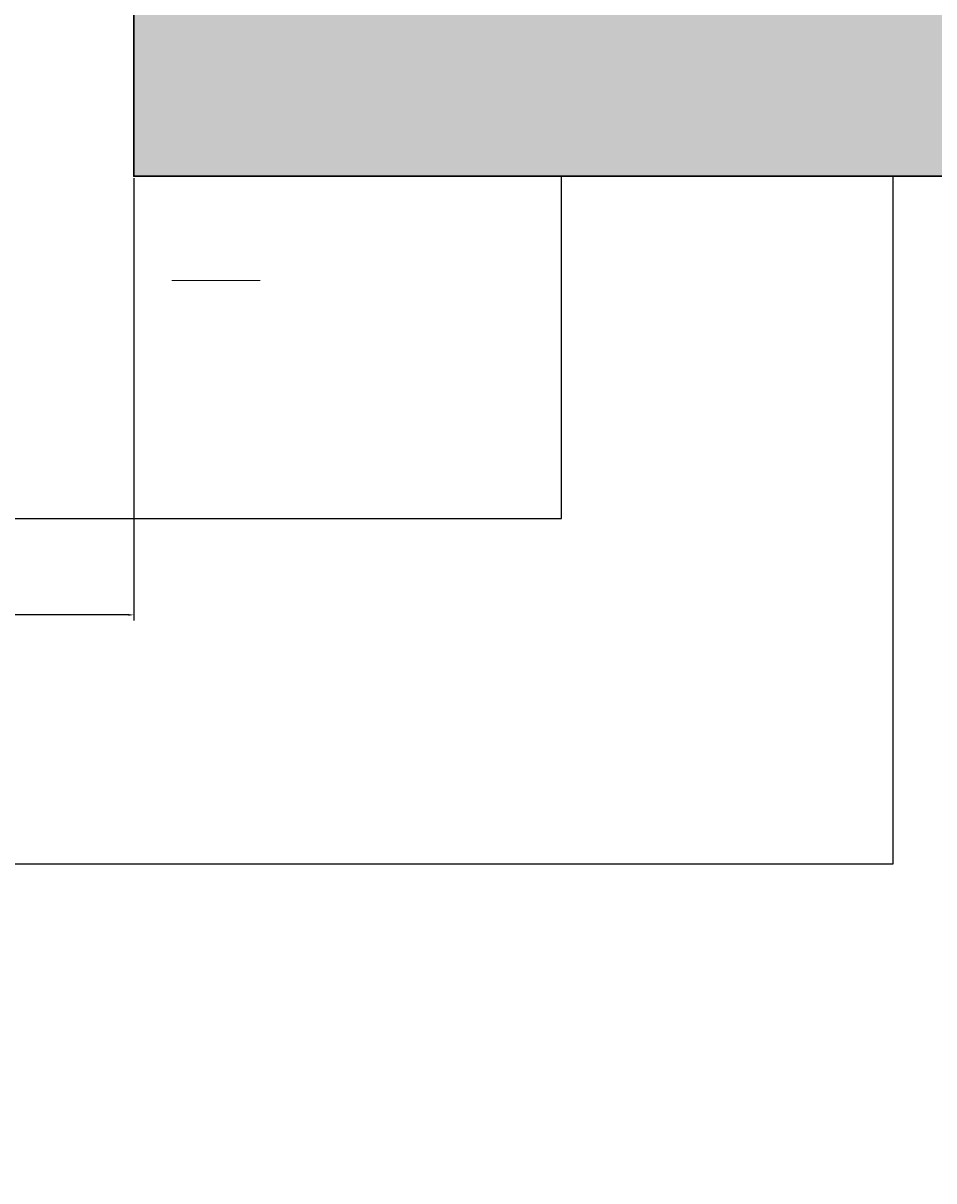
# Model space of a CAD drawing. Units: millimetres. Extents: x -8 to 285, y 5 to 221.
# Tile 13 of 30: x 47 to 76, y 113 to 150. Entities that reach past the tile are written whole.
import ezdxf

# ---------------------------------------------------------------- set-up
doc = ezdxf.new("R2010")
doc.units = ezdxf.units.MM
for name, color, linetype, lineweight in [('A-ANNO-DIMS', 2, 'Continuous', 18), ('E-ANNO-SYMB', 7, 'Continuous', 18), ('E-EQPM-PATT', 252, 'Continuous', 13), ('E-POWR-DC-LINK', 4, 'Continuous', 25), ('E-POWR-PV', 7, 'Continuous', 30)]:
    doc.layers.add(name, color=color, linetype=linetype, lineweight=lineweight)
doc.layers.add('E-POWR-DC-POS', color=30, linetype='Continuous', lineweight=25, true_color=0xf26722)
doc.styles.get("Standard").update_dxf_attribs({"font": 'arial.ttf'})
doc.dimstyles.get("Standard").update_dxf_attribs({"dimtxt": 0.18, "dimasz": 0.18, "dimexe": 0.18, "dimexo": 0.0625, "dimgap": 0.09, "dimtad": 0, "dimtih": 1, "dimtoh": 1, "dimdec": 4, "dimzin": 0, "dimdsep": 46, "dimtxsty": 'Standard', "dimcen": 0.09, "dimadec": 0, "dimazin": 0, "dimtfac": 1, "dimtdec": 4, "dimtofl": 0, "dimtmove": 0, "dimatfit": 3, "dimfxl": 1, "dimtolj": 1, "dimtzin": 0, "dimarcsym": 0})

# ---------------------------------------------------------------- blocks, each defined once
blk = doc.blocks.new('PV-MODULE-12V')
blk.add_lwpolyline([(0, 47), (37, 47), (37, 0), (0, 0)], close=True)
blk = doc.blocks.new('*D9')
at = {"layer": 'A-ANNO-DIMS', "color": 0, "lineweight": -2, "transparency": 16777216}
for p, q in [((6.672, 133.79), (6.672, 220.737)), ((270.919, 206.519), (270.919, 220.737)), ((6.852, 220.557), (138.33, 220.557)), ((270.739, 220.557), (139.262, 220.557))]:
    blk.add_line(p, q, dxfattribs=at)
at = {"layer": 'A-ANNO-DIMS', "color": 0, "transparency": 16777216}
for points in [[(6.852, 220.587), (6.852, 220.527), (6.672, 220.557)], [(270.739, 220.587), (270.739, 220.527), (270.919, 220.557)]]:
    blk.add_solid(points, dxfattribs=at)
at = {"layer": 'Defpoints', "color": 0, "transparency": 16777216}
for p in [(270.919, 220.557), (270.919, 206.457), (6.672, 133.727)]:
    blk.add_point(p, dxfattribs=at)
at = {"layer": 'A-ANNO-DIMS', "color": 0, "transparency": 16777216, "insert": (138.796, 220.557), "char_height": 0.18, "attachment_point": 5}
blk.add_mtext('\\A1;264.25', dxfattribs=at)
blk = doc.blocks.new('*D10')
at = {"layer": 'A-ANNO-DIMS', "color": 0, "lineweight": -2, "transparency": 16777216}
for p, q in [((145.103, 206.457), (-7.608, 206.457)), ((-7.428, 206.277), (-7.428, 113.161)), ((-7.428, 19.682), (-7.428, 112.797)), ((30.453, 19.502), (-7.608, 19.502))]:
    blk.add_line(p, q, dxfattribs=at)
at = {"layer": 'A-ANNO-DIMS', "color": 0, "transparency": 16777216}
for points in [[(-7.458, 206.277), (-7.398, 206.277), (-7.428, 206.457)], [(-7.458, 19.682), (-7.398, 19.682), (-7.428, 19.502)]]:
    blk.add_solid(points, dxfattribs=at)
at = {"layer": 'Defpoints', "color": 0, "transparency": 16777216}
for p in [(-7.428, 206.457), (145.165, 206.457), (30.516, 19.502)]:
    blk.add_point(p, dxfattribs=at)
at = {"layer": 'A-ANNO-DIMS', "color": 0, "transparency": 16777216, "insert": (-7.428, 112.979), "char_height": 0.18, "attachment_point": 5}
blk.add_mtext('\\A1;186.95', dxfattribs=at)
blk = doc.blocks.new('*D11')
at = {"layer": 'A-ANNO-DIMS', "color": 0, "lineweight": -2, "transparency": 16777216}
for p, q in [((6.853, 145.209), (6.853, 130.991)), ((50.572, 145.209), (50.572, 130.991)), ((7.033, 131.171), (28.316, 131.171)), ((50.392, 131.171), (29.109, 131.171))]:
    blk.add_line(p, q, dxfattribs=at)
at = {"layer": 'A-ANNO-DIMS', "color": 0, "transparency": 16777216}
for points in [[(7.033, 131.201), (7.033, 131.141), (6.853, 131.171)], [(50.392, 131.201), (50.392, 131.141), (50.572, 131.171)]]:
    blk.add_solid(points, dxfattribs=at)
at = {"layer": 'Defpoints', "color": 0, "transparency": 16777216}
for p in [(6.853, 145.271), (50.572, 145.271), (6.853, 131.171)]:
    blk.add_point(p, dxfattribs=at)
at = {"layer": 'A-ANNO-DIMS', "color": 0, "transparency": 16777216, "insert": (28.713, 131.171), "char_height": 0.18, "attachment_point": 5}
blk.add_mtext('\\A1;43.72', dxfattribs=at)

msp = doc.modelspace()

# ---------------------------------------------------------------- hatches: boundary and pattern name
at = {"layer": 'E-EQPM-PATT'}
h = msp.add_hatch(color=256, dxfattribs=at)
h.set_gradient(color2=(0, 0, 0), tint=1)
h.paths.add_polyline_path([(6.8535, 192.2715), (6.8535, 145.2715), (43.8535, 145.2715), (43.8535, 192.2715)])
h.paths.add_polyline_path([(37.8535, 186.2715), (37.8535, 151.2715), (12.8535, 151.2715), (12.8535, 186.2715)], flags=0)
h.paths.add_polyline_path([(50.5716, 145.2715), (87.5716, 145.2715), (87.5716, 192.2715), (50.5716, 192.2715)])
h.paths.add_polyline_path([(56.5716, 186.2715), (81.5716, 186.2715), (81.5716, 151.2715), (56.5716, 151.2715)], flags=0)
h.paths.add_polyline_path([(37.8535, 176.7715), (37.8535, 186.2715), (25.3535, 186.2715), (25.3535, 176.7715)], flags=0)
h.paths.add_polyline_path([(37.8535, 176.7715), (37.8535, 186.2715), (12.8535, 186.2715), (12.8535, 176.7715)], flags=0)
h.paths.add_polyline_path([(25.3535, 160.7715), (37.8535, 160.7715), (37.8535, 186.2715), (25.3535, 186.2715)], flags=0)
h.paths.add_polyline_path([(12.8535, 151.2715), (37.8535, 151.2715), (37.8535, 186.2715), (12.8535, 186.2715)], flags=16)
h.paths.add_polyline_path([(56.5716, 186.2715), (56.5716, 160.7715), (81.5716, 160.7715), (81.5716, 186.2715)], flags=0)
h.paths.add_polyline_path([(56.5716, 151.2715), (81.5716, 151.2715), (81.5716, 186.2715), (56.5716, 186.2715)], flags=16)

# ---------------------------------------------------------------- linework, layer by layer
at = {"layer": 'E-ANNO-SYMB'}
msp.add_line((51.7951, 141.9255), (54.6346, 141.9255), dxfattribs=at)
at = {"layer": 'E-POWR-DC-LINK'}
msp.add_lwpolyline([(29.8062, 145.2715), (29.8062, 134.2715), (64.3247, 134.2715), (64.3247, 145.2715)], dxfattribs=at)
at = {"layer": 'E-POWR-DC-POS'}
msp.add_lwpolyline([(74.9801, 145.2715), (74.9801, 123.1618), (17.279, 123.1618), (17.279, 54.6776), (40.1717, 54.6776), (40.1717, 67.9064)], dxfattribs=at)

# ---------------------------------------------------------------- block references
at = {"layer": 'E-POWR-PV'}
msp.add_blockref('PV-MODULE-12V', (50.5711, 145.271), dxfattribs=at)

# ---------------------------------------------------------------- dimensions: what is measured, and where the dimension line sits
at = {"layer": 'A-ANNO-DIMS'}
dim = msp.add_linear_dim(base=(270.9192, 220.5568), p1=(6.6725, 133.7273), p2=(270.9192, 206.4568), dimstyle='Standard', override={"dimdec": 2, "dimlfac": 1, "dimrnd": 0, "dimzin": 0, "dimdsep": 46, "dimlunit": 2}, dxfattribs=at)
dim.commit()
dim.dimension.update_dxf_attribs({"geometry": '*D9', "text_midpoint": (138.7958, 220.5568)})
for base, p1, p2, angle, picture, middle in [((-7.4275, 206.4568), (30.516, 19.502), (145.1651, 206.4568), 90, '*D10', (-7.4275, 112.9794)), ((6.8535, 131.1715), (50.5716, 145.2715), (6.8535, 145.2715), 180, '*D11', (28.7125, 131.1715))]:
    dim = msp.add_linear_dim(base=base, p1=p1, p2=p2, angle=angle, dimstyle='Standard', override={"dimdec": 2, "dimlfac": 1, "dimrnd": 0, "dimzin": 0, "dimdsep": 46, "dimlunit": 2}, dxfattribs=at)
    dim.commit()
    dim.dimension.update_dxf_attribs({"geometry": picture, "text_midpoint": middle})

doc.saveas('drawing.dxf')
